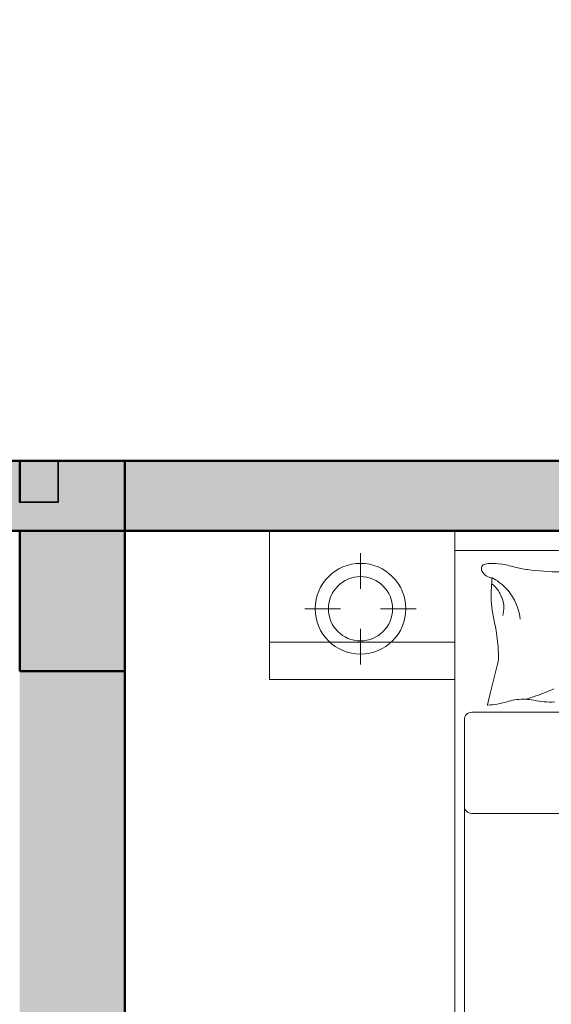
# Model space of a CAD drawing. Units: inches. Extents: x -7 to 1228, y -146 to 1091.
# Tile 29 of 88: x 634 to 680, y 446 to 531. Entities that reach past the tile are written whole.
import ezdxf

# ---------------------------------------------------------------- set-up
doc = ezdxf.new("R2010")
doc.units = ezdxf.units.IN
for name, color, linetype, lineweight in [('A-COLS', 6, 'Continuous', 35), ('A-FURN', 8, 'Continuous', 18), ('A-WALL', 7, 'Continuous', 50), ('A-WALL-PATT', 251, 'Continuous', 13)]:
    doc.layers.add(name, color=color, linetype=linetype, lineweight=lineweight)
doc.styles.add('DIM_FONT', font='SIMPLEX.shx', dxfattribs={"width": 0.8})

# ---------------------------------------------------------------- blocks, each defined once
blk = doc.blocks.new('A$C4F634EDD')
for p, q in [((0, 2.6295), (0, 2.2295)), ((0.5, 2.6295), (0, 2.6295)), ((0.5, 2.6295), (2.3, 2.6295)), ((0.5, 0.5295), (0.5, 2.6295)), ((0.5, 2.2295), (0.5, 2.6295)), ((0.5, 2.5771), (2.3, 2.5771)), ((0.2457, 2.5697), (0.2457, 2.4733)), ((0.0957, 2.4197), (0.192, 2.4197)), ((0.2994, 2.4197), (0.3957, 2.4197)), ((0.2457, 2.366), (0.2457, 2.2697)), ((0, 2.3301), (0.5, 2.3301)), ((0.5953, 2.1912), (0.616, 2.2738)), ((0, 2.2295), (0.5, 2.2295)), ((0.5878, 2.1612), (0.5953, 2.1912)), ((1.5035, 2.141), (0.5458, 2.141)), ((0.5258, 2.121), (0.5258, 0.5617)), ((0.5458, 1.8684), (1.5653, 1.8684))]:
    blk.add_line(p, q)
for radius in [0.1222, 0.0865]:
    blk.add_circle((0.2457, 2.4197), radius)
for centre, radius, start, end in [((0.5848, 2.5274), 0.0131, 101.2724, 206.5805), ((0.6036, 2.5368), 0.0342, 206.5805, 265.5998), ((0.5999, 2.4516), 0.0904, 90, 101.2724), ((0.5999, 2.3808), 0.1611, 81.5628, 90), ((0.5788, 2.2388), 0.3048, 74.256, 81.5628), ((0.7272, 2.7653), 0.2422, 254.256, 262.4531), ((0.7851, 3.2019), 0.6827, 262.4531, 270), ((1.0898, 2.4496), 0.4918, 173.7676, 180), ((0.5368, 2.3783), 0.1399, 45.0976, 62.7964), ((0.5462, 2.4142), 0.0899, 41.4429, 53.7359), ((0.5741, 2.4389), 0.0526, 25.3551, 41.4429), ((0.5368, 2.3783), 0.1399, 27.3988, 45.0976), ((0.8019, 2.4496), 0.204, 180, 189.6844), ((0.4851, 2.3967), 0.1511, 21.8149, 25.3551), ((0.4345, 2.3765), 0.2056, 18.7799, 21.8149), ((0.576, 2.4246), 0.0562, 0, 18.7799), ((0.5368, 2.3783), 0.1399, 16.515, 27.3988), ((1.4703, 2.5637), 0.882, 189.6844, 192.1984), ((0.5406, 2.4246), 0.0915, 345.3149, 0), ((0.5368, 2.3783), 0.1399, 5.6311, 16.515), ((0.2982, 2.3103), 0.3171, 8.0051, 12.1984), ((-0.0401, 2.2627), 0.6588, 2.6649, 8.0051), ((0.5503, 2.2902), 0.0677, 345.9548, 2.6649), ((0.473, 2.8815), 0.7387, 291.6577, 293.4844), ((0.6807, 2.0561), 0.1197, 96.4341, 107.3864), ((0.6836, 2.0301), 0.1459, 78.4414, 96.4341), ((0.473, 2.8815), 0.7387, 287.1982, 289.428), ((0.473, 2.8815), 0.7387, 289.428, 291.6577), ((0.5887, 2.1609), 0.000917, 165.9551, 274.0829), ((0.5695, 2.4301), 0.2708, 274.0829, 279.4841), ((0.5763, 2.3896), 0.2297, 279.4841, 287.3864), ((0.759, 2.3985), 0.2301, 258.4414, 272.7491), ((0.5458, 2.121), 0.02, 90, 180), ((0.5458, 1.8884), 0.02, 180, 270)]:
    blk.add_arc(centre, radius, start, end)
at = {"style": 'DIM_FONT', "width": 0.8, "flags": 9}
for tag, p in [('YSIZE', (0.5, 2.6295)), ('XSIZE', (0.5, 2.6295)), ('XSIZE', (2.2985, 2.6295)), ('YSIZE', (2.2985, 2.6295))]:
    blk.add_attdef(tag, p, '', height=0.0005, dxfattribs=at)

msp = doc.modelspace()

# ---------------------------------------------------------------- hatches: boundary and pattern name
at = {"layer": 'A-COLS'}
h = msp.add_hatch(color=256, dxfattribs=at)
h.dxf.hatch_style = 1
h.paths.add_polyline_path([(643, 475), (634, 475), (634, 489.454), (637.289, 489.454), (637.289, 493), (643, 493)])
h = msp.add_hatch(color=256, dxfattribs=at)
h.dxf.hatch_style = 1
h.paths.add_polyline_path([(637.289, 489.454), (637.289, 493), (634, 493), (634, 489.454)])
at = {"layer": 'A-WALL-PATT'}
h = msp.add_hatch(color=256, dxfattribs=at)
h.dxf.hatch_style = 1
h.paths.add_polyline_path([(69, 568), (60, 568), (60, 493), (63.289, 493), (69, 493)])
h.paths.add_polyline_path([(69, 662.405), (60, 662.405), (60, 586), (69, 586)], flags=17)
h.paths.add_polyline_path([(69, 723), (184, 723), (184, 734), (179, 734), (179, 728), (69, 728), (69, 741.623), (60, 741.623), (60, 698.405), (69, 698.405)], flags=17)
h.paths.add_polyline_path([(69, 782), (231, 782), (231, 728), (231, 723), (231, 586), (236, 586), (236, 787), (69, 787), (69, 800.126), (60, 800.126), (60, 765.623), (69, 765.623)])
h.paths.add_polyline_path([(184, 842), (189, 842), (189, 848), (173, 848), (173, 842), (179, 842), (179, 787), (184, 787)])
h.paths.add_polyline_path([(118.22, 69), (69, 69), (69, 60), (118.22, 60)])
h.paths.add_polyline_path([(227, 69), (154.22, 69), (154.22, 60), (227, 60)])
h.paths.add_polyline_path([(236, 60), (232.711, 60), (227, 60), (227, 36), (236, 36)])
h.paths.add_polyline_path([(389, 60), (380, 60), (380, 36), (389, 36)])
h.paths.add_polyline_path([(384, 181), (380, 181), (380, 115), (380, 78), (384, 78)])
h.paths.add_polyline_path([(380, 115), (334.547, 115), (334.547, 109), (380, 109)])
h.paths.add_polyline_path([(274.547, 115), (236, 115), (236, 201), (232.711, 201), (231, 201), (231, 78), (236, 78), (236, 109), (274.547, 109)])
h.paths.add_polyline_path([(69, 123), (60, 123), (60, 78), (69, 78)])
h.paths.add_polyline_path([(69, 201), (60, 201), (60, 159), (69, 159)])
h.paths.add_polyline_path([(143, 219), (69, 219), (69, 213), (143, 213)], flags=17)
h.paths.add_polyline_path([(189, 219), (184, 219), (184, 274), (231, 274), (231, 219), (236, 219), (236, 279), (184, 279), (184, 297), (179, 297), (179, 279), (69, 279), (69, 290.912), (60, 290.912), (60, 262.179), (69, 262.179), (69, 274), (179, 274), (179, 219), (173, 219), (173, 213), (189, 213)])
h.paths.add_polyline_path([(69, 238.179), (60, 238.179), (60, 219), (69, 219)], flags=17)
h.paths.add_polyline_path([(69, 333), (60, 333), (60, 314.912), (69, 314.912), (69, 316.965)])
h.paths.add_polyline_path([(190, 338), (184, 338), (69, 338), (69, 333), (179, 333), (179, 327), (184, 327), (184, 333.021), (190, 333.046)])
h.paths.add_polyline_path([(69, 386.806), (60, 386.806), (60, 351), (69, 351)])
h.paths.add_polyline_path([(69, 475), (60, 475), (60, 422.806), (69, 422.806)])
h.paths.add_polyline_path([(236, 475), (231, 475), (231, 351.238), (236, 351.238)])
h.paths.add_polyline_path([(384, 475), (380, 475), (380, 362), (384, 362)])
h.paths.add_polyline_path([(547, 307), (439, 307), (439, 356), (445, 356), (445, 362), (433, 362), (433, 307), (380, 307), (380, 244), (380, 241), (384, 241), (384, 301), (433, 301), (433, 277), (439, 277), (439, 301), (547, 301)])
h.paths.add_polyline_path([(547, 241), (439, 241), (439, 247), (433, 247), (433, 235), (547, 235)])
h.paths.add_polyline_path([(450, 69), (440.286, 69), (424.889, 69), (389, 69), (389, 60), (450, 60)])
h.paths.add_polyline_path([(547, 69), (486, 69), (486, 60), (547, 60)])
h.paths.add_polyline_path([(556, 148.268), (547, 148.268), (547, 78), (556, 78)])
h.paths.add_polyline_path([(556, 223), (547, 223), (547, 195), (547, 184.268), (556, 184.268)])
h.paths.add_polyline_path([(556, 311.192), (547, 311.192), (547, 273.075), (556, 273.075)])
h.paths.add_polyline_path([(556, 344), (552.711, 344), (547, 344), (547, 335.192), (556, 335.192)])
h.paths.add_polyline_path([(556, 249.075), (547, 249.075), (547, 241), (556, 241)])
h.paths.add_polyline_path([(547, 362), (475, 362), (475, 356), (547, 356)], flags=0)
h.paths.add_polyline_path([(556, 399.621), (547, 399.621), (547, 362), (556, 362)])
h.paths.add_polyline_path([(556, 475), (547, 475), (547, 435.621), (556, 435.621)])
h.paths.add_polyline_path([(547, 493), (389, 493), (389, 487), (547, 487)])
h.paths.add_polyline_path([(380, 493), (278, 493), (278, 487), (380, 487)])
h.paths.add_polyline_path([(227, 493), (69, 493), (69, 487), (227, 487)])
h.paths.add_polyline_path([(643, 122.445), (634, 122.445), (634, 78), (643, 78)])
h.paths.add_polyline_path([(702.5, 69), (692.786, 69), (677.389, 69), (643, 69), (643, 60), (702.5, 60)])
h.paths.add_polyline_path([(798, 69), (738.5, 69), (738.5, 60), (798, 60)])
h.paths.add_polyline_path([(807, 60), (803.711, 60), (798, 60), (798, 36), (807, 36)])
h.paths.add_polyline_path([(807, 109), (846.751, 109), (846.751, 115), (807, 115), (807, 159), (802, 159), (802, 78), (807, 78)])
h.paths.add_polyline_path([(807, 201), (802, 201), (802, 195), (807, 195)])
h.paths.add_polyline_path([(643, 201), (634, 201), (634, 158.445), (643, 158.445)])
h.paths.add_polyline_path([(756, 225), (751, 225), (751, 219), (643, 219), (643, 213), (756, 213)])
h.paths.add_polyline_path([(643, 240.848), (634, 240.848), (634, 219), (643, 219)])
h.paths.add_polyline_path([(643, 274), (643, 288.629), (634, 288.629), (634, 264.848), (643, 264.848)])
h.paths.add_polyline_path([(802, 279), (756, 279), (756, 297), (751, 297), (751, 279), (643, 279), (643, 274), (751, 274), (751, 255), (756, 255), (756, 274), (802, 274)])
h.paths.add_polyline_path([(807, 333), (803.711, 333), (802, 333), (802, 279), (802, 274), (802, 219), (807, 219)])
h.paths.add_polyline_path([(956, 182), (951, 182), (951, 115), (906.751, 115), (906.751, 109), (951, 109), (951, 78), (956, 78)])
h.paths.add_polyline_path([(960, 60), (951, 60), (951, 36), (960, 36)])
h.paths.add_polyline_path([(1021, 69), (1005.781, 69), (960, 69), (960, 60), (1021, 60)])
h.paths.add_polyline_path([(956, 224), (951, 224), (951, 218), (956, 218)])
h.paths.add_polyline_path([(956, 302), (1004, 302), (1004, 278), (1010, 278), (1010, 302), (1118, 302), (1118, 290.809), (1127, 290.809), (1127, 326.968), (1118, 326.968), (1118, 320.966), (1118, 307), (1010, 307), (1010, 356), (1016, 356), (1016, 362), (1004, 362), (1004, 307), (951, 307), (951, 244), (951, 242), (954.289, 242), (956, 242)])
h.paths.add_polyline_path([(643, 333), (634, 333), (634, 312.629), (643, 312.629), (643, 316.965)])
h.paths.add_polyline_path([(756, 338), (643, 338), (643, 333), (751, 333), (751, 327), (756, 327)])
h.paths.add_polyline_path([(643, 388), (634, 388), (634, 351), (643, 351)])
h.paths.add_polyline_path([(807, 357), (802, 357), (802, 351), (807, 351)])
h.paths.add_polyline_path([(807, 475), (802, 475), (802, 393), (807, 393)])
h.paths.add_polyline_path([(643, 475), (634, 475), (634, 424), (643, 424)])
h.paths.add_polyline_path([(798, 493), (643, 493), (643, 487), (798, 487)])
h.paths.add_polyline_path([(634, 493), (556, 493), (556, 487), (634, 487)])
h.paths.add_polyline_path([(813, 493), (807, 493), (807, 487), (813, 487)])
h.paths.add_polyline_path([(951, 493), (849, 493), (849, 487), (951, 487)])
h.paths.add_polyline_path([(956, 484), (951, 484), (951, 374), (956, 374)])
h.paths.add_polyline_path([(1109, 493), (969, 493), (969, 487), (1109, 487)])
h.paths.add_polyline_path([(1127, 484), (1118, 484), (1118, 450.641), (1127, 450.641)])
h.paths.add_polyline_path([(1127, 414.641), (1118, 414.641), (1118, 365), (1127, 365)])
h.paths.add_polyline_path([(1109, 362), (1046, 362), (1046, 356), (1109, 356)], flags=17)
h.paths.add_polyline_path([(1127, 356), (1123.454, 356), (1118, 356), (1118, 350.968), (1127, 350.968)], flags=0)
h.paths.add_polyline_path([(1127, 266.809), (1118, 266.809), (1118, 262.361), (1118, 242), (1127, 242)], flags=17)
h.paths.add_polyline_path([(1118, 242), (1010, 242), (1010, 248), (1004, 248), (1004, 237), (1118, 237)])
h.paths.add_polyline_path([(1127, 224), (1118, 224), (1118, 170), (1127, 170)])
h.paths.add_polyline_path([(1127, 134), (1118, 134), (1118, 78), (1127, 78)])
h.paths.add_polyline_path([(1118, 69), (1057, 69), (1057, 60), (1118, 60)])
h.paths.add_polyline_path([(227, 571.546), (227, 574), (69, 574), (69, 568), (227, 568)])
h.paths.add_polyline_path([(380, 571.546), (380, 574), (278, 574), (278, 568), (380, 568)])
h.paths.add_polyline_path([(242, 574), (236, 574), (236, 568), (242, 568)])
h.paths.add_polyline_path([(547, 571.546), (547, 574), (389, 574), (389, 568), (547, 568)])
h.paths.add_polyline_path([(384, 733), (380, 733), (380, 586), (384, 586)])
h.paths.add_polyline_path([(556, 646), (634, 646), (634, 655), (547, 655), (547, 586), (556, 586)])
h.paths.add_polyline_path([(634, 574), (556, 574), (556, 568), (634, 568)])
h.paths.add_polyline_path([(643, 655), (634, 655), (634, 586), (643, 586)])
h.paths.add_polyline_path([(798, 574), (643, 574), (643, 568), (798, 568)])
h.paths.add_polyline_path([(643, 663.854), (634, 663.854), (634, 655), (643, 655)])
h.paths.add_polyline_path([(556, 676.967), (547, 676.967), (547, 655), (556, 655)])
h.paths.add_polyline_path([(556, 733), (547, 733), (547, 712.967), (556, 712.967)])
h.paths.add_polyline_path([(643, 710), (634, 710), (634, 699.854), (643, 699.854)])
h.paths.add_polyline_path([(807, 668), (802, 668), (802, 586), (807, 586)])
h.paths.add_polyline_path([(951, 574), (849, 574), (849, 568), (951, 568)])
h.paths.add_polyline_path([(956, 691), (951, 691), (951, 577), (956, 577)])
h.paths.add_polyline_path([(1109, 574), (969, 574), (969, 568), (1109, 568)])
h.paths.add_polyline_path([(1127, 643.403), (1118, 643.403), (1118, 577), (1127, 577)])
h.paths.add_polyline_path([(1127, 568), (1123.454, 568), (1118, 568), (1118, 493), (1127, 493)])
h.paths.add_polyline_path([(1127, 733), (1118, 733), (1118, 679.403), (1127, 679.403)])
h.paths.add_polyline_path([(1127, 777.348), (1118, 777.348), (1118, 770.035), (1118, 751), (1127, 751)], flags=17)
h.paths.add_polyline_path([(1118, 751), (1010, 751), (1010, 757), (1004, 757), (1004, 745), (1118, 745)])
h.paths.add_polyline_path([(956, 811), (1004, 811), (1004, 787), (1010, 787), (1010, 811), (1017.874, 811), (1017.874, 811.627, -0.414214), (1018.247, 812), (1031.978, 812, -0.414214), (1032.351, 811.627), (1032.351, 811), (1118, 811), (1118, 801.348), (1127, 801.348), (1127, 834.685), (1118, 834.685), (1118, 830.238), (1118, 817), (1010, 817), (1010, 866), (1016, 866), (1016, 872), (1004, 872), (1004, 817), (956, 817), (956, 866), (951, 866), (951, 751), (954.289, 751), (956, 751)])
h.paths.add_polyline_path([(1118, 872), (1046, 872), (1046, 866), (1118, 866)], flags=17)
h.paths.add_polyline_path([(1127, 924.711), (1118, 924.711), (1118, 884), (1127, 884)])
h.paths.add_polyline_path([(1127, 866), (1123.711, 866), (1118, 866), (1118, 858.685), (1127, 858.685)], flags=17)
h.paths.add_polyline_path([(956, 983), (951, 983), (951, 952), (807, 952), (807, 983), (802, 983), (802, 902), (807, 902), (807, 946), (951, 946), (951, 884), (956, 884)])
h.paths.add_polyline_path([(807, 842), (802, 842), (802, 787), (756, 787), (756, 806), (751, 806), (751, 787), (643, 787), (643, 782), (751, 782), (751, 764), (756, 764), (756, 782), (802, 782), (802, 728), (807, 728)])
h.paths.add_polyline_path([(756, 848), (643, 848), (643, 842), (751, 842), (751, 836), (756, 836)])
h.paths.add_polyline_path([(756, 734), (751, 734), (751, 728), (643, 728), (643, 723), (756, 723)])
h.paths.add_polyline_path([(643, 749.791), (634, 749.791), (634, 728), (637.289, 728), (643, 728)])
h.paths.add_polyline_path([(643, 805.405), (634, 805.405), (634, 773.791), (643, 773.791)])
h.paths.add_polyline_path([(643, 896.663), (634, 896.663), (634, 860), (637.289, 860), (643, 860)])
h.paths.add_polyline_path([(643, 842), (634, 842), (634, 829.405), (643, 829.405)])
h.paths.add_polyline_path([(643, 983), (634, 983), (634, 932.663), (643, 932.663)])
h.paths.add_polyline_path([(1127, 983), (1118, 983), (1118, 960.711), (1127, 960.711)])
h.paths.add_polyline_path([(1118, 1001), (1077.525, 1001), (1077.525, 992), (1118, 992)])
h.paths.add_polyline_path([(1041.525, 1001), (960, 1001), (960, 992), (1041.525, 992)])
h.paths.add_polyline_path([(960, 1025), (951, 1025), (951, 1001), (954.289, 1001), (960, 1001)])
h.paths.add_polyline_path([(807, 1025), (798, 1025), (798, 1001), (807, 1001)])
h.paths.add_polyline_path([(798, 1001), (738.5, 1001), (738.5, 992), (798, 992)])
h.paths.add_polyline_path([(702.5, 1001), (643, 1001), (643, 992), (702.5, 992)])
h.paths.add_polyline_path([(547, 1001), (499.113, 1001), (499.113, 992), (547, 992)])
h.paths.add_polyline_path([(463.113, 1001), (389, 1001), (389, 992), (463.113, 992)])
h.paths.add_polyline_path([(389, 1025), (380, 1025), (380, 1022), (380, 1001), (383.289, 1001), (389, 1001)])
h.paths.add_polyline_path([(236, 1025), (227, 1025), (227, 1001), (236, 1001)])
h.paths.add_polyline_path([(236, 983), (231, 983), (231, 860), (236, 860)])
h.paths.add_polyline_path([(274.547, 952), (236, 952), (236, 946), (274.547, 946)])
h.paths.add_polyline_path([(380, 952), (334.547, 952), (334.547, 946), (380, 946)])
h.paths.add_polyline_path([(384, 983), (380, 983), (380, 884), (383.289, 884), (384, 884)])
h.paths.add_polyline_path([(227, 1001), (155.012, 1001), (155.012, 992), (162.875, 992), (227, 992)])
h.paths.add_polyline_path([(119.012, 1001), (69, 1001), (69, 992), (119.012, 992)])
h.paths.add_polyline_path([(69, 983), (60, 983), (60, 922.987), (69, 922.987)])
h.paths.add_polyline_path([(69, 886.987), (60, 886.987), (60, 860), (63.289, 860), (69, 860)])
h.paths.add_polyline_path([(143, 848), (69, 848), (69, 842), (143, 842)])

# ---------------------------------------------------------------- linework, layer by layer
at = {"layer": 'A-COLS'}
msp.add_lwpolyline([(634, 493), (637.289, 493), (637.289, 489.454), (634, 489.454)], close=True, dxfattribs=at)
at = {"layer": 'A-WALL'}
for p, q in [((813, 493), (556, 493)), ((634, 493), (643, 493)), ((634, 489.454), (634, 493)), ((643, 338), (643, 493)), ((643, 493), (643, 475)), ((643, 493), (643, 60)), ((813, 487), (556, 487)), ((634, 475), (634, 487)), ((643, 475), (634, 475))]:
    msp.add_line(p, q, dxfattribs=at)

# ---------------------------------------------------------------- block references
at = {"layer": 'A-FURN', "xscale": 31.78426361944092, "yscale": 31.78426361944092, "zscale": 31.78426361944092}
msp.add_blockref('A$C4F634EDD', (655.397, 403.423), dxfattribs=at)

doc.saveas('drawing.dxf')
